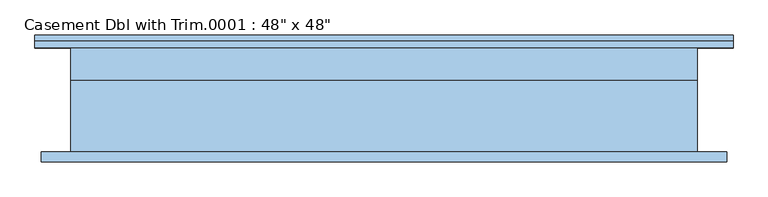
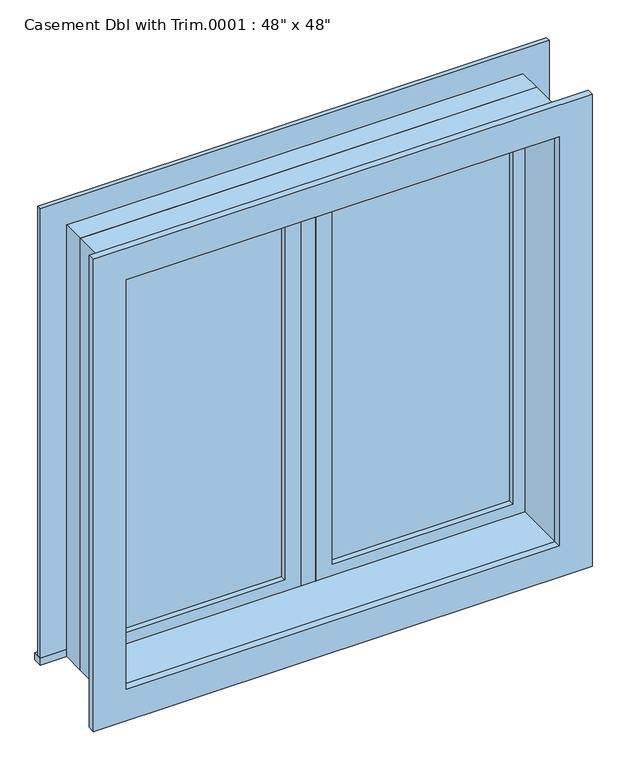
"""IFC4 building model written with IfcOpenShell, lengths in millimetres: window geometry."""

from ifc_helpers import new_model, si_unit, frame, origin, place, context, project, spatial, polyline, outline, extrude, source, transform, mapped, element, save


def window_0862ab64(model_context):
    return source(origin(), model_context, "Body", "SweptSolid", [
        extrude(outline(polyline([(63.5, 85.725), (546.1, 85.725), (546.1, 73.025), (63.5, 73.025), (63.5, 85.725)])), frame((0.0, 0.0, 977.9), z_axis=(0.0, 0.0, 1.0), x_axis=(1.0, 0.0, 0.0)), (0.0, 0.0, 1.0), 1092.2),
        extrude(outline(polyline([(2114.55, 19.05), (933.45, 19.05), (933.45, 590.55), (2114.55, 590.55), (2114.55, 19.05)]), holes=[polyline([(2070.1, 63.5), (2070.1, 546.1), (977.9, 546.1), (977.9, 63.5), (2070.1, 63.5)])]), frame((0.0, 57.15, 0.0), z_axis=(0.0, 1.0, 0.0), x_axis=(0.0, 0.0, 1.0)), (0.0, 0.0, 1.0), 44.45),
        extrude(outline(polyline([(19.05, 57.15), (-19.05, 57.15), (-19.05, 120.65), (19.05, 120.65), (19.05, 57.15)])), frame((0.0, 0.0, 933.45), z_axis=(0.0, 0.0, 1.0), x_axis=(1.0, 0.0, 0.0)), (0.0, 0.0, 1.0), 1181.1),
        extrude(outline(polyline([(-679.45, 146.05), (679.45, 146.05), (679.45, 120.65), (-679.45, 120.65), (-679.45, 146.05)])), frame((0.0, 0.0, 914.4), z_axis=(0.0, 0.0, 1.0), x_axis=(1.0, 0.0, 0.0)), (0.0, 0.0, 1.0), 19.05),
        extrude(outline(polyline([(2114.55, -590.55), (2114.55, 590.55), (933.45, 590.55), (933.45, 679.45), (2203.45, 679.45), (2203.45, -679.45), (933.45, -679.45), (933.45, -590.55), (2114.55, -590.55)])), frame((0.0, 120.65, 0.0), z_axis=(0.0, 1.0, 0.0), x_axis=(0.0, 0.0, 1.0)), (0.0, 0.0, 1.0), 12.7),
        extrude(outline(polyline([(2190.75, 666.75), (2190.75, -666.75), (857.25, -666.75), (857.25, 666.75), (2190.75, 666.75)]), holes=[polyline([(2101.85, 577.85), (946.15, 577.85), (946.15, -577.85), (2101.85, -577.85), (2101.85, 577.85)])]), frame((0.0, -101.6, 0.0), z_axis=(0.0, 1.0, 0.0), x_axis=(0.0, 0.0, 1.0)), (0.0, 0.0, 1.0), 19.05),
        extrude(outline(polyline([(-63.5, 73.025), (-546.1, 73.025), (-546.1, 85.725), (-63.5, 85.725), (-63.5, 73.025)])), frame((0.0, 0.0, 977.9), z_axis=(0.0, 0.0, 1.0), x_axis=(1.0, 0.0, 0.0)), (0.0, 0.0, 1.0), 1092.2),
        extrude(outline(polyline([(2114.55, -590.55), (933.45, -590.55), (933.45, -19.05), (2114.55, -19.05), (2114.55, -590.55)]), holes=[polyline([(2070.1, -546.1), (2070.1, -63.5), (977.9, -63.5), (977.9, -546.1), (2070.1, -546.1)])]), frame((0.0, 57.15, 0.0), z_axis=(0.0, 1.0, 0.0), x_axis=(0.0, 0.0, 1.0)), (0.0, 0.0, 1.0), 44.45),
        extrude(outline(polyline([(2133.6, -609.6), (914.4, -609.6), (914.4, 609.6), (2133.6, 609.6), (2133.6, -609.6)]), holes=[polyline([(2101.85, -577.85), (2101.85, 577.85), (946.15, 577.85), (946.15, -577.85), (2101.85, -577.85)])]), frame((0.0, -82.55, 0.0), z_axis=(0.0, 1.0, 0.0), x_axis=(0.0, 0.0, 1.0)), (0.0, 0.0, 1.0), 139.7),
        extrude(outline(polyline([(2133.6, 609.6), (2133.6, -609.6), (914.4, -609.6), (914.4, 609.6), (2133.6, 609.6)]), holes=[polyline([(2114.55, 590.55), (933.45, 590.55), (933.45, -590.55), (2114.55, -590.55), (2114.55, 590.55)])]), frame((0.0, 57.15, 0.0), z_axis=(0.0, 1.0, 0.0), x_axis=(0.0, 0.0, 1.0)), (0.0, 0.0, 1.0), 63.5),
    ])


if __name__ == "__main__":
    model = new_model("IFC4")
    model_context = context("Model", 3, world=origin())
    ifc_project = project(units=[si_unit("LENGTHUNIT", "METRE", prefix="MILLI")], contexts=[model_context])
    site = spatial("IfcSite", under=ifc_project)
    building = spatial("IfcBuilding", under=site)
    placement = place(None, origin())
    window_shape = window_0862ab64(model_context)
    element("IfcWindow", 1, ObjectType="Casement Dbl with Trim.0001 : 48\" x 48\"", at=placement, inside=building, context=model_context, shape_type="MappedRepresentation", body=[
        mapped(window_shape, transform((0.0, 0.0, 0.0), x_axis=(1.0, 0.0, 0.0), y_axis=(0.0, 1.0, 0.0), z_axis=(0.0, 0.0, 1.0))),
    ])
    save(model, "model.ifc")

# Revit data of these elements
# Type "Casement Dbl with Trim.0001 : 48\" x 48\""
#   Type Mark = "13"
#   Construction Type Id = "GSP4R"
#   Assembly Code = "B2020100"
#   Analytic Construction = "1/8 in Pilkington single glazing"
#   Visual Light Transmittance = 0.9
#   Solar Heat Gain Coefficient = 0.78
#   Heat Transfer Coefficient (U) = 0.6496 BTU/(h·ft²·°F)
#   Height = 4' - 0"
#   Default Sill Height = 3' - 0"
#   Trim Projection - Ext. = 0' - 0 1/2"
#   Trim Projection - Int. = 0' - 0 3/4"
#   Trim Width - Exterior = 0' - 3 1/2"
#   Trim Width - Interior = 0' - 3 1/2"
#   Width = 4' - 0"
#   Window Inset = 0' - 0 3/4"
#   Define Thermal Properties by = 1
#   Glass Pane Material = Glass
#   Sash Material = Sash
#   Trim Exterior Material = Trim
#   Trim Interior Material = Trim
#   Wall Closure = (empty or 0)
# Element 1 (IfcWindow, "Casement Dbl with Trim.0001 : 48\" x 48\"")
#   Materials on its faces: "Sash", "Trim", "Glass"
# Materials
#   "Glass": class "Glass", colour RGB 0 128 192, transparency 0.75, Description = "Soda Lime Glass", Cost = 0
#   "Sash": class "Wood", colour RGB 224 178 126, transparency 0
#   "Trim": class "Wood", colour RGB 224 178 126, transparency 0
